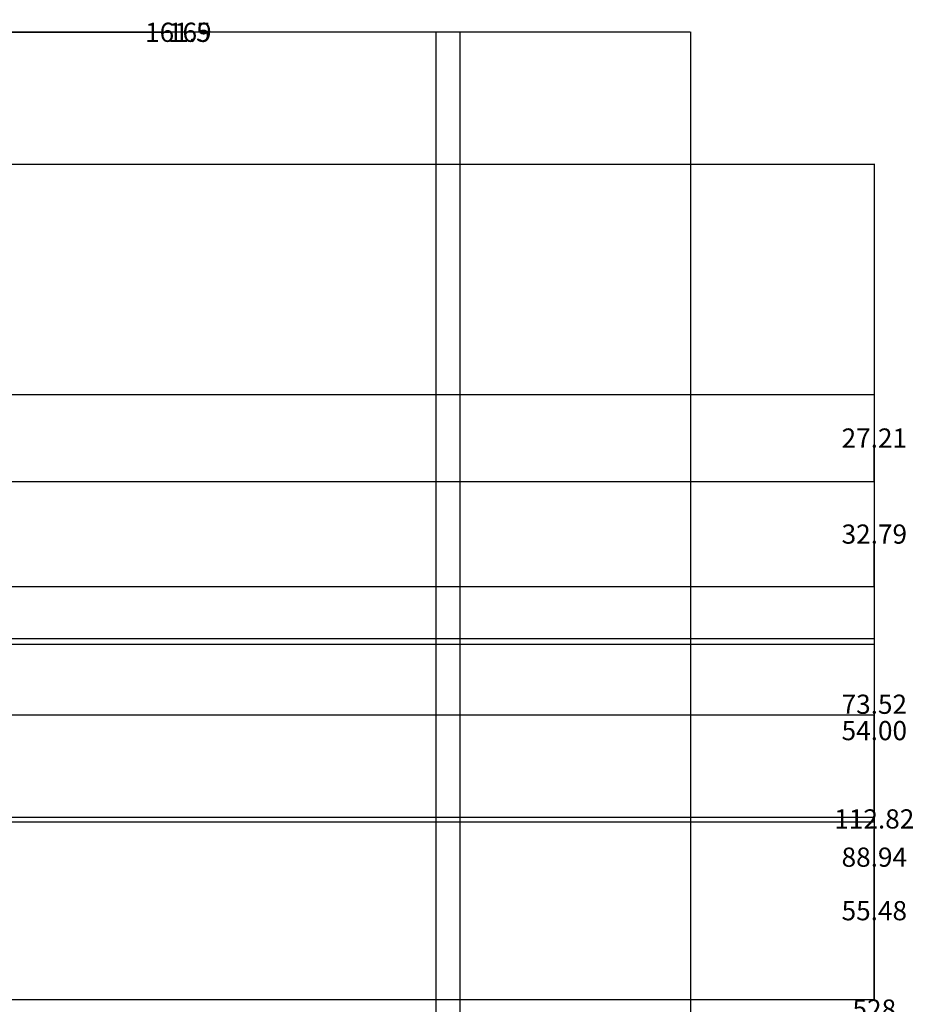
# Model space of a CAD drawing. Units: inches. Extents: x 148 to 1080, y 89 to 707.
# Tile 12 of 12: x 797 to 1077, y 399 to 707. Entities that reach past the tile are written whole.
import ezdxf

# ---------------------------------------------------------------- set-up
doc = ezdxf.new("R2010")
doc.units = ezdxf.units.IN
doc.header["$MEASUREMENT"] = 0
doc.layers.add('A-ANNO-DIMS', color=2, linetype='Continuous', lineweight=18)
doc.styles.get("Standard").update_dxf_attribs({"font": 'arial.ttf'})
doc.dimstyles.get("Standard").update_dxf_attribs({"dimtxt": 6, "dimasz": 0.18, "dimexe": 0.18, "dimexo": 0.0625, "dimgap": 0.09, "dimtad": 0, "dimtih": 1, "dimtoh": 1, "dimdec": 0, "dimzin": 0, "dimdsep": 46, "dimlunit": 3, "dimtxsty": 'Standard', "dimcen": 0.09, "dimadec": 0, "dimazin": 0, "dimtfac": 1, "dimtdec": 0, "dimtofl": 0, "dimtmove": 0, "dimatfit": 3, "dimfxl": 1, "dimtolj": 1, "dimtzin": 0, "dimarcsym": 0})

# ---------------------------------------------------------------- blocks, each defined once
blk = doc.blocks.new('*D1')
at = {"layer": 'A-ANNO-DIMS', "color": 0, "lineweight": -2, "transparency": 16777216}
for p, q in [((215.02, 662.01), (215.02, 703.28)), ((215.2, 703.1), (604.32, 703.1)), ((1006.77, 703.1), (617.65, 703.1)), ((1006.95, 338.01), (1006.95, 703.28))]:
    blk.add_line(p, q, dxfattribs=at)
at = {"layer": 'A-ANNO-DIMS', "color": 0, "transparency": 16777216}
for points in [[(215.2, 703.13), (215.2, 703.07), (215.02, 703.1)], [(1006.77, 703.13), (1006.77, 703.07), (1006.95, 703.1)]]:
    blk.add_solid(points, dxfattribs=at)
at = {"layer": 'Defpoints', "color": 0, "transparency": 16777216}
for p in [(1006.95, 703.1), (215.02, 661.95), (1006.95, 337.95)]:
    blk.add_point(p, dxfattribs=at)
at = {"layer": 'A-ANNO-DIMS', "color": 0, "transparency": 16777216, "insert": (610.98, 703.1), "char_height": 6, "attachment_point": 5}
blk.add_mtext('\\A1;792', dxfattribs=at)
blk = doc.blocks.new('*D18')
at = {"layer": 'A-ANNO-DIMS', "color": 0, "lineweight": -2, "transparency": 16777216}
for p, q in [((635.08, 661.95), (1064.5, 661.95)), ((1064.32, 661.77), (1064.32, 401.1)), ((1064.32, 134.13), (1064.32, 394.79)), ((1007.01, 133.95), (1064.5, 133.95))]:
    blk.add_line(p, q, dxfattribs=at)
at = {"layer": 'A-ANNO-DIMS', "color": 0, "transparency": 16777216}
for points in [[(1064.29, 661.77), (1064.35, 661.77), (1064.32, 661.95)], [(1064.29, 134.13), (1064.35, 134.13), (1064.32, 133.95)]]:
    blk.add_solid(points, dxfattribs=at)
at = {"layer": 'Defpoints', "color": 0, "transparency": 16777216}
for p in [(635.02, 661.95), (1064.32, 661.95), (1006.95, 133.95)]:
    blk.add_point(p, dxfattribs=at)
at = {"layer": 'A-ANNO-DIMS', "color": 0, "transparency": 16777216, "insert": (1064.32, 397.95), "char_height": 6, "attachment_point": 5}
blk.add_mtext('\\A1;528', dxfattribs=at)
blk = doc.blocks.new('*D36')
at = {"layer": 'A-ANNO-DIMS', "color": 0, "lineweight": -2, "transparency": 16777216}
for p, q in [((765.95, 241.16), (765.95, 703.28)), ((766.13, 703.1), (844.01, 703.1)), ((934.77, 703.1), (856.89, 703.1)), ((934.95, 272.01), (934.95, 703.28))]:
    blk.add_line(p, q, dxfattribs=at)
at = {"layer": 'A-ANNO-DIMS', "color": 0, "transparency": 16777216}
for points in [[(766.13, 703.13), (766.13, 703.07), (765.95, 703.1)], [(934.77, 703.13), (934.77, 703.07), (934.95, 703.1)]]:
    blk.add_solid(points, dxfattribs=at)
at = {"layer": 'Defpoints', "color": 0, "transparency": 16777216}
for p in [(934.95, 703.1), (934.95, 271.95), (765.95, 241.1)]:
    blk.add_point(p, dxfattribs=at)
at = {"layer": 'A-ANNO-DIMS', "color": 0, "transparency": 16777216, "insert": (850.45, 703.1), "char_height": 6, "attachment_point": 5}
blk.add_mtext('\\A1;169', dxfattribs=at)
blk = doc.blocks.new('*D37')
at = {"layer": 'A-ANNO-DIMS', "color": 0, "lineweight": -2, "transparency": 16777216}
for p, q in [((765.95, 241.16), (765.95, 703.28)), ((766.13, 703.1), (836.75, 703.1)), ((927.28, 703.1), (856.66, 703.1)), ((927.46, 240.26), (927.46, 703.28))]:
    blk.add_line(p, q, dxfattribs=at)
at = {"layer": 'A-ANNO-DIMS', "color": 0, "transparency": 16777216}
for points in [[(766.13, 703.13), (766.13, 703.07), (765.95, 703.1)], [(927.28, 703.13), (927.28, 703.07), (927.46, 703.1)]]:
    blk.add_solid(points, dxfattribs=at)
at = {"layer": 'Defpoints', "color": 0, "transparency": 16777216}
for p in [(927.46, 703.1), (765.95, 241.1), (927.46, 240.2)]:
    blk.add_point(p, dxfattribs=at)
at = {"layer": 'A-ANNO-DIMS', "color": 0, "transparency": 16777216, "insert": (846.7, 703.1), "char_height": 6, "attachment_point": 5}
blk.add_mtext('\\A1;161.5', dxfattribs=at)
blk = doc.blocks.new('*D51')
at = {"layer": 'A-ANNO-DIMS', "color": 0, "lineweight": -2, "transparency": 16777216}
for p, q in [((707.08, 511.95), (1064.5, 511.95)), ((1064.32, 511.77), (1064.32, 488.1)), ((1064.32, 458.13), (1064.32, 481.79)), ((695.08, 457.95), (1064.5, 457.95))]:
    blk.add_line(p, q, dxfattribs=at)
at = {"layer": 'A-ANNO-DIMS', "color": 0, "transparency": 16777216}
for points in [[(1064.29, 511.77), (1064.35, 511.77), (1064.32, 511.95)], [(1064.29, 458.13), (1064.35, 458.13), (1064.32, 457.95)]]:
    blk.add_solid(points, dxfattribs=at)
at = {"layer": 'Defpoints', "color": 0, "transparency": 16777216}
for p in [(707.02, 511.95), (695.02, 457.95), (1064.32, 457.95)]:
    blk.add_point(p, dxfattribs=at)
at = {"layer": 'A-ANNO-DIMS', "color": 0, "transparency": 16777216, "insert": (1064.32, 484.95), "char_height": 6, "attachment_point": 5}
blk.add_mtext('\\A1;54.00', dxfattribs=at)
blk = doc.blocks.new('*D90')
at = {"layer": 'A-ANNO-DIMS', "color": 0, "lineweight": -2, "transparency": 16777216}
for p, q in [((527.08, 489.89), (1064.5, 489.89)), ((1064.32, 489.71), (1064.32, 448.57)), ((1064.32, 401.13), (1064.32, 442.27)), ((527.08, 400.95), (1064.5, 400.95))]:
    blk.add_line(p, q, dxfattribs=at)
at = {"layer": 'A-ANNO-DIMS', "color": 0, "transparency": 16777216}
for points in [[(1064.29, 489.71), (1064.35, 489.71), (1064.32, 489.89)], [(1064.29, 401.13), (1064.35, 401.13), (1064.32, 400.95)]]:
    blk.add_solid(points, dxfattribs=at)
at = {"layer": 'Defpoints', "color": 0, "transparency": 16777216}
for p in [(527.02, 489.89), (527.02, 400.95), (1064.32, 400.95)]:
    blk.add_point(p, dxfattribs=at)
at = {"layer": 'A-ANNO-DIMS', "color": 0, "transparency": 16777216, "insert": (1064.32, 445.42), "char_height": 6, "attachment_point": 5}
blk.add_mtext('\\A1;88.94', dxfattribs=at)
blk = doc.blocks.new('*D91')
at = {"layer": 'A-ANNO-DIMS', "color": 0, "lineweight": -2, "transparency": 16777216}
for p, q in [((479.08, 513.77), (1064.5, 513.77)), ((1064.32, 513.59), (1064.32, 460.51)), ((1064.32, 401.13), (1064.32, 454.21)), ((479.08, 400.95), (1064.5, 400.95))]:
    blk.add_line(p, q, dxfattribs=at)
at = {"layer": 'A-ANNO-DIMS', "color": 0, "transparency": 16777216}
for points in [[(1064.29, 513.59), (1064.35, 513.59), (1064.32, 513.77)], [(1064.29, 401.13), (1064.35, 401.13), (1064.32, 400.95)]]:
    blk.add_solid(points, dxfattribs=at)
at = {"layer": 'Defpoints', "color": 0, "transparency": 16777216}
for p in [(479.02, 513.77), (479.02, 400.95), (1064.32, 400.95)]:
    blk.add_point(p, dxfattribs=at)
at = {"layer": 'A-ANNO-DIMS', "color": 0, "transparency": 16777216, "insert": (1064.32, 457.36), "char_height": 6, "attachment_point": 5}
blk.add_mtext('\\A1;112.82', dxfattribs=at)
blk = doc.blocks.new('*D92')
at = {"layer": 'A-ANNO-DIMS', "color": 0, "lineweight": -2, "transparency": 16777216}
for p, q in [((389.08, 456.43), (1064.5, 456.43)), ((1064.32, 456.25), (1064.32, 431.84)), ((1064.32, 401.13), (1064.32, 425.53)), ((389.08, 400.95), (1064.5, 400.95))]:
    blk.add_line(p, q, dxfattribs=at)
at = {"layer": 'A-ANNO-DIMS', "color": 0, "transparency": 16777216}
for points in [[(1064.29, 456.25), (1064.35, 456.25), (1064.32, 456.43)], [(1064.29, 401.13), (1064.35, 401.13), (1064.32, 400.95)]]:
    blk.add_solid(points, dxfattribs=at)
at = {"layer": 'Defpoints', "color": 0, "transparency": 16777216}
for p in [(389.02, 456.43), (1064.32, 456.43), (389.02, 400.95)]:
    blk.add_point(p, dxfattribs=at)
at = {"layer": 'A-ANNO-DIMS', "color": 0, "transparency": 16777216, "insert": (1064.32, 428.69), "char_height": 6, "attachment_point": 5}
blk.add_mtext('\\A1;55.48', dxfattribs=at)
blk = doc.blocks.new('*D93')
at = {"layer": 'A-ANNO-DIMS', "color": 0, "lineweight": -2, "transparency": 16777216}
for p, q in [((389.08, 529.95), (1064.5, 529.95)), ((1064.32, 529.77), (1064.32, 496.34)), ((1064.32, 456.61), (1064.32, 490.03)), ((389.08, 456.43), (1064.5, 456.43))]:
    blk.add_line(p, q, dxfattribs=at)
at = {"layer": 'A-ANNO-DIMS', "color": 0, "transparency": 16777216}
for points in [[(1064.29, 529.77), (1064.35, 529.77), (1064.32, 529.95)], [(1064.29, 456.61), (1064.35, 456.61), (1064.32, 456.43)]]:
    blk.add_solid(points, dxfattribs=at)
at = {"layer": 'Defpoints', "color": 0, "transparency": 16777216}
for p in [(389.02, 529.95), (1064.32, 529.95), (389.02, 456.43)]:
    blk.add_point(p, dxfattribs=at)
at = {"layer": 'A-ANNO-DIMS', "color": 0, "transparency": 16777216, "insert": (1064.32, 493.19), "char_height": 6, "attachment_point": 5}
blk.add_mtext('\\A1;73.52', dxfattribs=at)
blk = doc.blocks.new('*D94')
at = {"layer": 'A-ANNO-DIMS', "color": 0, "lineweight": -2, "transparency": 16777216}
for p, q in [((389.08, 562.74), (1064.5, 562.74)), ((1064.32, 562.56), (1064.32, 549.5)), ((1064.32, 530.13), (1064.32, 543.19)), ((389.08, 529.95), (1064.5, 529.95))]:
    blk.add_line(p, q, dxfattribs=at)
at = {"layer": 'A-ANNO-DIMS', "color": 0, "transparency": 16777216}
for points in [[(1064.29, 562.56), (1064.35, 562.56), (1064.32, 562.74)], [(1064.29, 530.13), (1064.35, 530.13), (1064.32, 529.95)]]:
    blk.add_solid(points, dxfattribs=at)
at = {"layer": 'Defpoints', "color": 0, "transparency": 16777216}
for p in [(389.02, 562.74), (1064.32, 562.74), (389.02, 529.95)]:
    blk.add_point(p, dxfattribs=at)
at = {"layer": 'A-ANNO-DIMS', "color": 0, "transparency": 16777216, "insert": (1064.32, 546.34), "char_height": 6, "attachment_point": 5}
blk.add_mtext('\\A1;32.79', dxfattribs=at)
blk = doc.blocks.new('*D95')
at = {"layer": 'A-ANNO-DIMS', "color": 0, "lineweight": -2, "transparency": 16777216}
for p, q in [((389.08, 589.95), (1064.5, 589.95)), ((1064.32, 589.77), (1064.32, 579.44)), ((1064.32, 562.92), (1064.32, 573.24)), ((389.08, 562.74), (1064.5, 562.74))]:
    blk.add_line(p, q, dxfattribs=at)
at = {"layer": 'A-ANNO-DIMS', "color": 0, "transparency": 16777216}
for points in [[(1064.29, 589.77), (1064.35, 589.77), (1064.32, 589.95)], [(1064.29, 562.92), (1064.35, 562.92), (1064.32, 562.74)]]:
    blk.add_solid(points, dxfattribs=at)
at = {"layer": 'Defpoints', "color": 0, "transparency": 16777216}
for p in [(389.02, 589.95), (1064.32, 589.95), (389.02, 562.74)]:
    blk.add_point(p, dxfattribs=at)
at = {"layer": 'A-ANNO-DIMS', "color": 0, "transparency": 16777216, "insert": (1064.32, 576.34), "char_height": 6, "attachment_point": 5}
blk.add_mtext('\\A1;27.21', dxfattribs=at)

msp = doc.modelspace()

# ---------------------------------------------------------------- dimensions: what is measured, and where the dimension line sits
at = {"layer": 'A-ANNO-DIMS'}
for base, p1, p2, override, picture, middle in [((1006.9492, 703.0974), (215.0199, 661.9474), (1006.9492, 337.9474), {"dimdec": 0, "dimlfac": 1, "dimrnd": 0, "dimzin": 0, "dimdsep": 46, "dimlunit": 2}, '*D1', (610.9845, 703.0974)), ((934.9492, 703.0974), (765.9474, 241.0996), (934.9492, 271.9474), {"dimdec": 0, "dimlfac": 1, "dimrnd": 0, "dimzin": 0, "dimdsep": 46, "dimlunit": 2}, '*D36', (850.4483, 703.0974)), ((927.4587, 703.0974), (765.9474, 241.0996), (927.4587, 240.1966), {"dimdec": 1, "dimlfac": 1, "dimrnd": 0, "dimzin": 0, "dimdsep": 46, "dimlunit": 2}, '*D37', (846.703, 703.0974))]:
    dim = msp.add_linear_dim(base=base, p1=p1, p2=p2, dimstyle='Standard', override=override, dxfattribs=at)
    dim.commit()
    dim.dimension.update_dxf_attribs({"geometry": picture, "text_midpoint": middle})
for base, p1, p2, override, picture, middle in [((1064.325, 661.9474), (1006.9492, 133.9474), (635.0199, 661.9474), {"dimdec": 0, "dimlfac": 1, "dimrnd": 0, "dimzin": 0, "dimdsep": 46, "dimlunit": 2}, '*D18', (1064.325, 397.9474)), ((1064.325, 589.9474), (389.0199, 562.736), (389.0199, 589.9474), {"dimdec": 2, "dimlfac": 1, "dimrnd": 0, "dimzin": 0, "dimdsep": 46, "dimlunit": 2}, '*D95', (1064.325, 576.3417)), ((1064.325, 562.736), (389.0199, 529.9474), (389.0199, 562.736), {"dimdec": 2, "dimlfac": 1, "dimrnd": 0, "dimzin": 0, "dimdsep": 46, "dimlunit": 2}, '*D94', (1064.325, 546.3417)), ((1064.325, 529.9474), (389.0199, 456.4274), (389.0199, 529.9474), {"dimdec": 2, "dimlfac": 1, "dimrnd": 0, "dimzin": 0, "dimdsep": 46, "dimlunit": 2}, '*D93', (1064.325, 493.1874)), ((1064.325, 400.9474), (479.0199, 513.7706), (479.0199, 400.9474), {"dimdec": 2, "dimlfac": 1, "dimrnd": 0, "dimzin": 0, "dimdsep": 46, "dimlunit": 2}, '*D91', (1064.325, 457.359)), ((1064.325, 457.9474), (707.0199, 511.9474), (695.0199, 457.9474), {"dimdec": 2, "dimlfac": 1, "dimrnd": 0, "dimzin": 0, "dimdsep": 46, "dimlunit": 2}, '*D51', (1064.325, 484.9474)), ((1064.325, 400.9474), (527.0199, 489.89), (527.0199, 400.9474), {"dimdec": 2, "dimlfac": 1, "dimrnd": 0, "dimzin": 0, "dimdsep": 46, "dimlunit": 2}, '*D90', (1064.325, 445.4187)), ((1064.325, 456.4274), (389.0199, 400.9474), (389.0199, 456.4274), {"dimdec": 2, "dimlfac": 1, "dimrnd": 0, "dimzin": 0, "dimdsep": 46, "dimlunit": 2}, '*D92', (1064.325, 428.6874))]:
    dim = msp.add_linear_dim(base=base, p1=p1, p2=p2, angle=90, dimstyle='Standard', override=override, dxfattribs=at)
    dim.commit()
    dim.dimension.update_dxf_attribs({"geometry": picture, "text_midpoint": middle})

doc.saveas('drawing.dxf')
